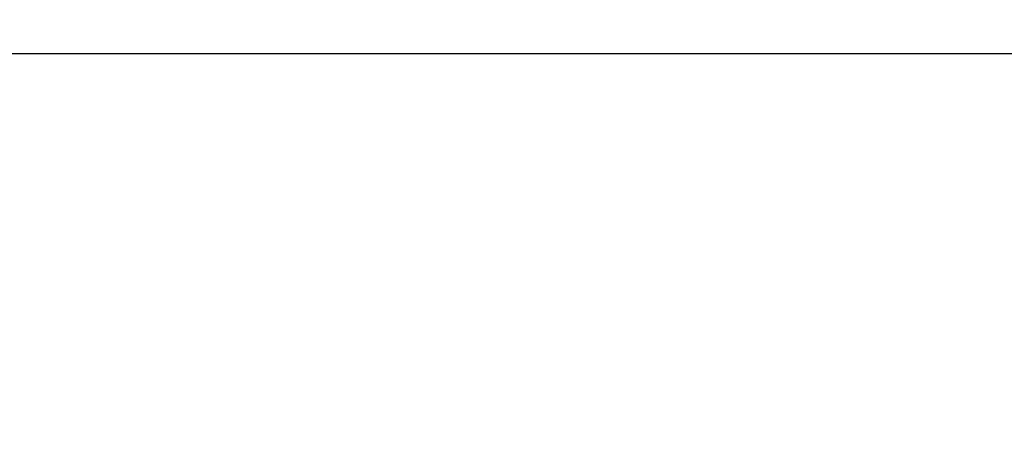
# Model space of a CAD drawing. Units: inches. Extents: x -36302355 to 648, y -221479757 to 75.
# Tile 36 of 37: x 227 to 341, y 26 to 75. Entities that reach past the tile are written whole.
import ezdxf

# ---------------------------------------------------------------- set-up
doc = ezdxf.new("R2010")
doc.units = ezdxf.units.IN
doc.header["$MEASUREMENT"] = 0
doc.layers.add('A-ANNO-DIMS', color=2, linetype='Continuous', lineweight=18)
doc.styles.get("Standard").update_dxf_attribs({"font": 'arial.ttf'})
doc.dimstyles.get("Standard").update_dxf_attribs({"dimtxt": 0.18, "dimasz": 0.18, "dimexe": 0.18, "dimexo": 0.0625, "dimgap": 0.09, "dimtad": 0, "dimtih": 1, "dimtoh": 1, "dimdec": 0, "dimzin": 0, "dimdsep": 46, "dimlunit": 3, "dimtxsty": 'Standard', "dimcen": 0.09, "dimadec": 0, "dimazin": 0, "dimtfac": 1, "dimtdec": 0, "dimtofl": 0, "dimtmove": 0, "dimatfit": 3, "dimfxl": 1, "dimtolj": 1, "dimtzin": 0, "dimarcsym": 0})

# ---------------------------------------------------------------- blocks, each defined once
blk = doc.blocks.new('*D4')
at = {"layer": 'A-ANNO-DIMS', "color": 0, "lineweight": -2, "transparency": 16777216}
for p, q in [((145.2, 25.04), (145.2, 71.11)), ((145.38, 70.93), (364.8, 70.93)), ((605.02, 70.93), (385.59, 70.93)), ((605.2, 25.04), (605.2, 71.11))]:
    blk.add_line(p, q, dxfattribs=at)
at = {"layer": 'A-ANNO-DIMS', "color": 0, "transparency": 16777216}
for points in [[(145.38, 70.96), (145.38, 70.9), (145.2, 70.93)], [(605.02, 70.96), (605.02, 70.9), (605.2, 70.93)]]:
    blk.add_solid(points, dxfattribs=at)
at = {"layer": 'Defpoints', "color": 0, "transparency": 16777216}
for p in [(605.2, 70.93), (145.2, 24.98), (605.2, 24.98)]:
    blk.add_point(p, dxfattribs=at)
at = {"layer": 'A-ANNO-DIMS', "color": 0, "transparency": 16777216, "insert": (375.2, 70.93), "char_height": 6, "attachment_point": 5}
blk.add_mtext('\\A1;38\'-4"', dxfattribs=at)

msp = doc.modelspace()

# ---------------------------------------------------------------- dimensions: what is measured, and where the dimension line sits
at = {"layer": 'A-ANNO-DIMS'}
dim = msp.add_linear_dim(base=(605.2, 70.93), p1=(145.2, 24.98), p2=(605.2, 24.98), dimstyle='Standard', override={"dimtxt": 6, "dimclrd": 0, "dimclre": 0, "dimclrt": 0}, dxfattribs=at)
dim.commit()
dim.dimension.update_dxf_attribs({"geometry": '*D4', "text_midpoint": (375.2, 70.93)})

doc.saveas('drawing.dxf')
